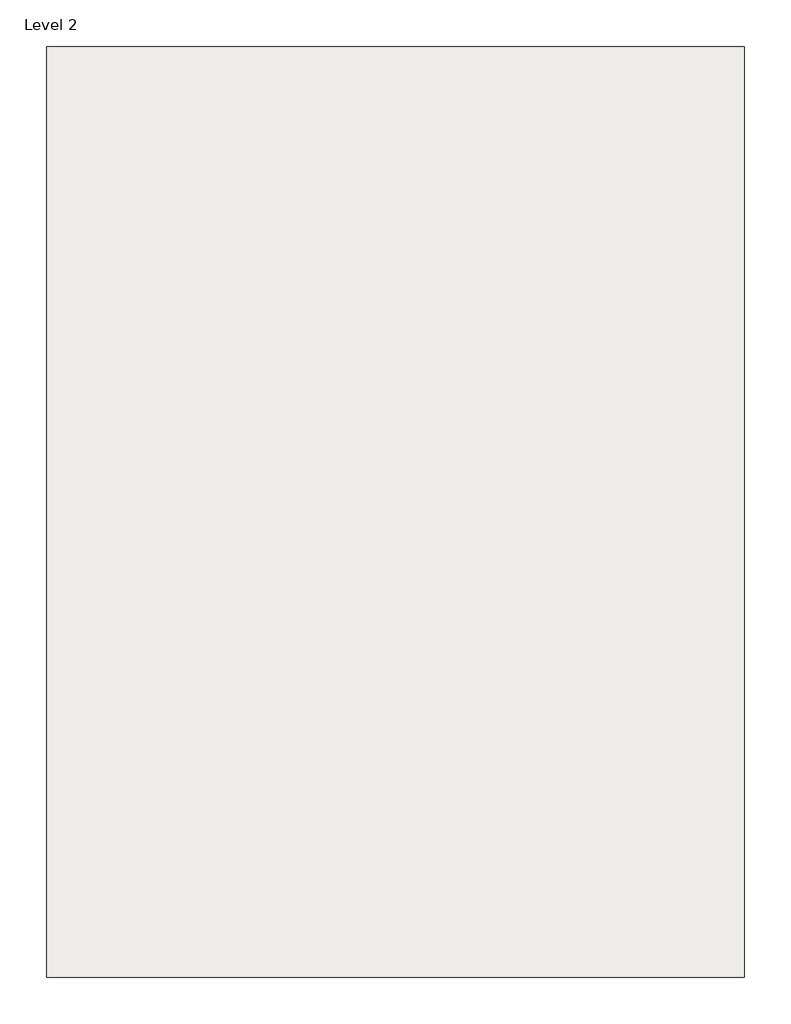
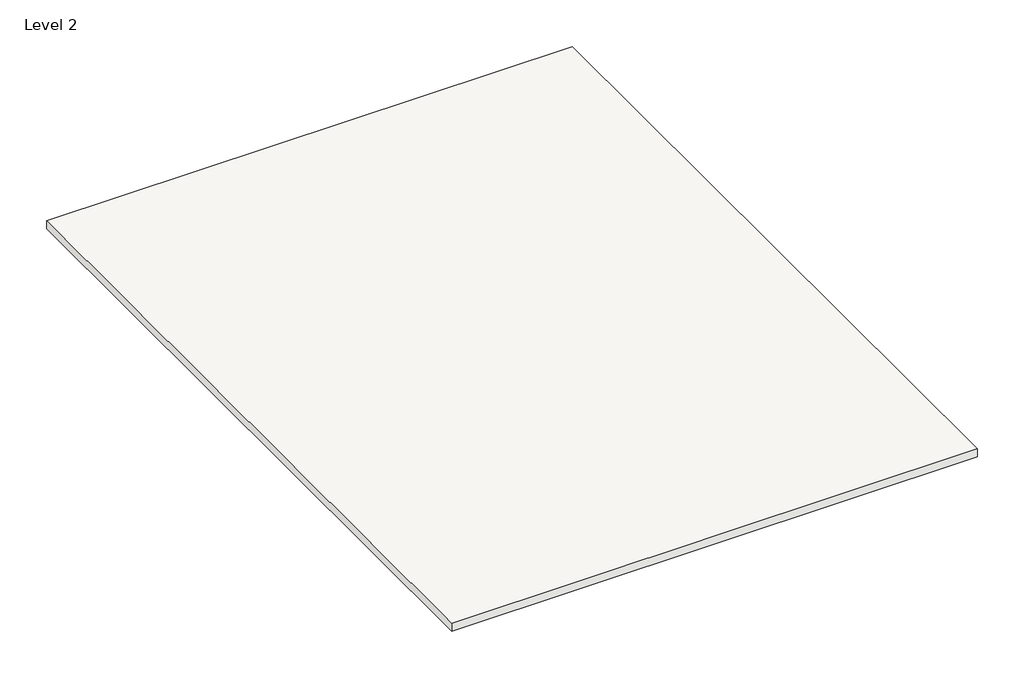
# One storey, incomplete: 1 roof.
"""IFC4 building model written with IfcOpenShell, lengths in millimetres."""

from ifc_helpers import new_model, si_unit, frame, origin, place, context, project, spatial, polyline, outline, extrude, element, save

model = new_model("IFC4")

# Units and contexts
model_context = context("Model", 3, world=origin())
ifc_project = project(units=[si_unit("LENGTHUNIT", "METRE", prefix="MILLI")], contexts=[model_context])

# Site, building, storey
site = spatial("IfcSite", under=ifc_project)
building = spatial("IfcBuilding", under=site)
storey = spatial("IfcBuildingStorey", under=building, Name="Level 2", Elevation=3048.0)

# Roof
placement = place(None, origin())
element("IfcRoof", 1, ObjectType="roof 6\"", at=placement, inside=storey, context=model_context, shape_type="SweptSolid", body=[
    extrude(outline(polyline([(-5709.2760342, 6447.2507456), (3828.4239658, 6447.2507456), (3828.4239658, -6278.1492544), (-5709.2760342, -6278.1492544), (-5709.2760342, 6447.2507456)])), frame((0.0, 0.0, 3048.0), z_axis=(0.0, 0.0, 1.0), x_axis=(1.0, 0.0, 0.0)), (0.0, 0.0, 1.0), 152.4),
])

save(model, "model.ifc")

# Revit data of these elements
# Type "roof 6\""
#   Assembly Code = "B1020"
#   Layers, outside or top first: 0' - 6" no material (function 1)
# Element 1 (IfcRoof, "roof 6\"")
#   built-in parameter 1001705 = 10.5 (stored number, unit not read)
#   built-in parameter 1001710 = 33615
#   Phase Created = New Construction
#   Materials on its faces: "Copper", "Default Roof", "Wood - Stained"
# Materials
#   "Copper": class "Metal", colour RGB 0 0 0, transparency 0, Description = "Copper, matte finish", Cost = 0
#   "Default Roof": colour RGB 88 101 114, transparency 0, Cost = 0
#   "Wood - Stained": class "Wood", colour RGB 224 178 126, transparency 0, Cost = 0
